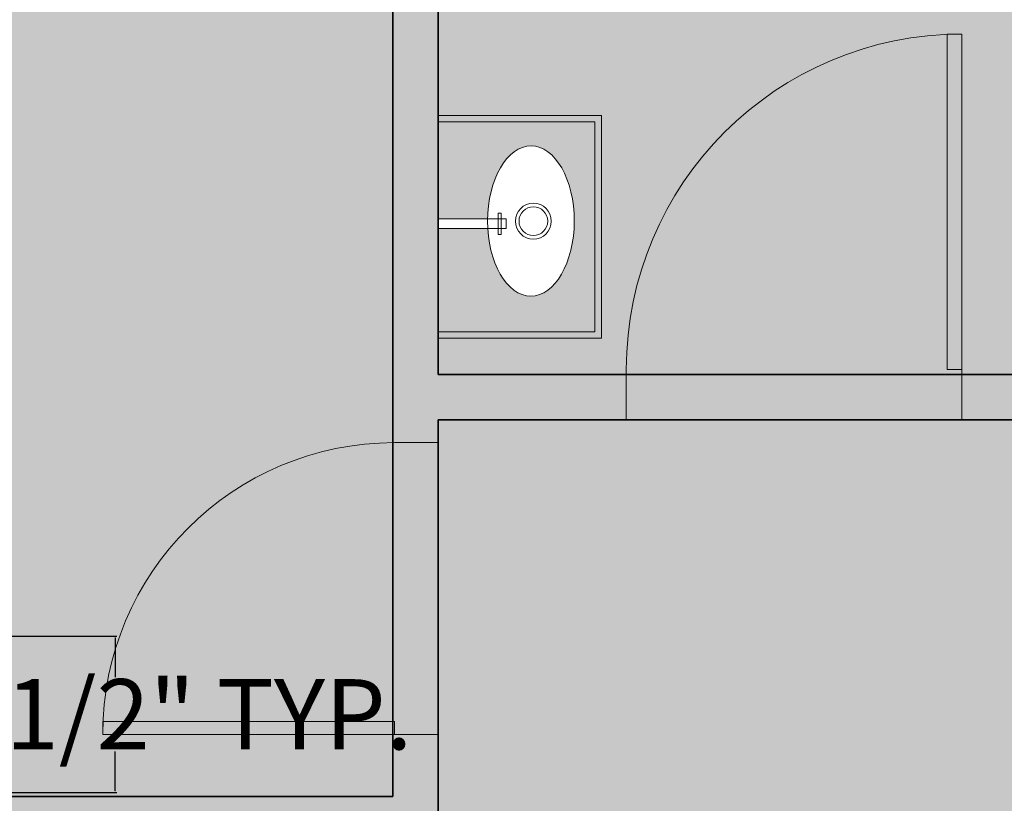
# Model space of a CAD drawing. Units: inches. Extents: x 1316 to 1777, y 813 to 1650.
# Tile 14 of 22: x 1469 to 1567, y 1434 to 1512. Entities that reach past the tile are written whole.
import ezdxf

# ---------------------------------------------------------------- set-up
doc = ezdxf.new("R2010")
doc.units = ezdxf.units.IN
doc.header["$MEASUREMENT"] = 0
for name, color, linetype, lineweight in [('A-ANNO-DIMS', 2, 'Continuous', 18), ('A-DOOR', 4, 'Continuous', 18), ('A-DOOR-PATT', 253, 'Continuous', 13), ('A-FLOR-FIXT', 8, 'Continuous', 18), ('A-FLOR-FIXT-PATT', 23, 'Continuous', 13), ('A-WALL-PATT', 250, 'Continuous', 13), ('walls', 250, 'Continuous', 35)]:
    doc.layers.add(name, color=color, linetype=linetype, lineweight=lineweight)
doc.layers.add('A-FLOR-PATT', color=254, linetype='Continuous', lineweight=13, true_color=0xfeeab9)
doc.styles.get("Standard").update_dxf_attribs({"font": 'arial.ttf'})
doc.dimstyles.get("Standard").update_dxf_attribs({"dimtxt": 7, "dimasz": 0.18, "dimexe": 0.18, "dimexo": 0.0625, "dimgap": 0.09, "dimtad": 0, "dimtih": 1, "dimtoh": 1, "dimzin": 0, "dimdsep": 46, "dimlunit": 3, "dimtxsty": 'Standard', "dimcen": 0.09, "dimadec": 0, "dimazin": 0, "dimtfac": 1, "dimtofl": 0, "dimtmove": 0, "dimatfit": 3, "dimfxl": 1, "dimtolj": 1, "dimtzin": 0, "dimarcsym": 0})

# ---------------------------------------------------------------- blocks, each defined once
blk = doc.blocks.new('*U15')
for p, q in [((0, 0), (-1e-16, -5.999999999999999)), ((40, -6e-16), (40, -6))]:
    blk.add_line(p, q)
blk.add_lwpolyline([(0, 0), (5.6e-15, 40), (1.750000000000007, 40), (1.749999999999998, -7e-16)], close=True)
blk.add_arc((0, 0), 40, 0, 90)
blk = doc.blocks.new('*D30')
at = {"layer": 'A-ANNO-DIMS', "color": 0, "lineweight": -2, "transparency": 16777216}
for p, q in [((1386.153353095512, 1434.699095169867), (1386.153353095512, 1422.57802783725)), ((1466.177135312958, 1434.699095169867), (1466.177135312958, 1422.57802783725)), ((1386.333353095512, 1422.75802783725), (1465.997135312959, 1422.75802783725)), ((1466.177135312958, 1422.75802783725), (1466.357135312958, 1422.75802783725))]:
    blk.add_line(p, q, dxfattribs=at)
at = {"layer": 'A-ANNO-DIMS', "color": 0, "transparency": 16777216}
for points in [[(1386.333353095512, 1422.78802783725), (1386.333353095512, 1422.72802783725), (1386.153353095512, 1422.75802783725)], [(1465.997135312959, 1422.78802783725), (1465.997135312959, 1422.72802783725), (1466.177135312958, 1422.75802783725)]]:
    blk.add_solid(points, dxfattribs=at)
at = {"layer": 'Defpoints', "color": 0, "transparency": 16777216}
for p in [(1386.153353095512, 1434.761595169867), (1466.177135312958, 1434.761595169867), (1466.177135312958, 1422.75802783725)]:
    blk.add_point(p, dxfattribs=at)
at = {"layer": 'A-ANNO-DIMS', "color": 0, "transparency": 16777216, "insert": (1518.078103935059, 1422.75802783725), "char_height": 7, "attachment_point": 5}
blk.add_mtext('\\A1;WARDROBE 6\'-8" TYP.', dxfattribs=at)
blk = doc.blocks.new('*D31')
at = {"layer": 'A-ANNO-DIMS', "color": 0, "lineweight": -2, "transparency": 16777216}
for p, q in [((1466.239635312959, 1450.329145456027), (1478.360702645576, 1450.329145456027)), ((1478.180702645576, 1450.149145456027), (1478.180702645576, 1446.257130203807)), ((1478.180702645576, 1434.941595169868), (1478.180702645576, 1438.833610422088)), ((1466.239635312959, 1434.761595169868), (1478.360702645576, 1434.761595169868))]:
    blk.add_line(p, q, dxfattribs=at)
at = {"layer": 'A-ANNO-DIMS', "color": 0, "transparency": 16777216}
for points in [[(1478.150702645576, 1450.149145456027), (1478.210702645576, 1450.149145456027), (1478.180702645576, 1450.329145456027)], [(1478.150702645576, 1434.941595169868), (1478.210702645576, 1434.941595169868), (1478.180702645576, 1434.761595169868)]]:
    blk.add_solid(points, dxfattribs=at)
at = {"layer": 'Defpoints', "color": 0, "transparency": 16777216}
for p in [(1466.177135312959, 1450.329145456027), (1478.180702645576, 1450.329145456027), (1466.177135312959, 1434.761595169868)]:
    blk.add_point(p, dxfattribs=at)
at = {"layer": 'A-ANNO-DIMS', "color": 0, "transparency": 16777216, "insert": (1478.180702645576, 1442.545370312947), "char_height": 7, "attachment_point": 5}
blk.add_mtext('\\A1;1\'-3 1/2" TYP.', dxfattribs=at)

msp = doc.modelspace()

# ---------------------------------------------------------------- hatches: boundary and pattern name
at = {"layer": 'A-DOOR-PATT'}
h = msp.add_hatch(color=256, dxfattribs=at)
h.dxf.hatch_style = 1
h.paths.add_polyline_path([(1440.064450217018, 1373.459281729462), (1411.195884528974, 1373.459281729462, 0.0109414287710455), (1411.168078720428, 1372.18876759644), (1440.064450217018, 1372.18876759644)])
h.paths.add_polyline_path([(1505.845136951899, 1441.821674157348), (1476.976571263855, 1441.821674157348, 0.0109414287710455), (1476.948765455309, 1440.551160024325), (1505.845136951899, 1440.551160024325)])
h.paths.add_polyline_path([(1510.345136951899, 1469.591483064839), (1505.989088495822, 1469.591483064839, 0.0012392441961977), (1505.845136951899, 1469.59112628206), (1505.845136951899, 1441.821674157348), (1505.989088495822, 1441.821674157348), (1505.989088495822, 1440.551160024325), (1510.345136951899, 1440.551160024325)])
at = {"layer": 'A-FLOR-FIXT-PATT'}
h = msp.add_hatch(color=256, dxfattribs=at)
h.dxf.hatch_style = 1
edge = h.paths.add_edge_path(flags=0)
edge.add_line((1525.946608831446, 1501.531624720906), (1510.345136951899, 1501.531624720906))
edge.add_line((1510.345136951899, 1501.531624720906), (1510.345136951899, 1491.869370531834))
edge.add_line((1510.345136951899, 1491.869370531834), (1515.276633424269, 1491.869370531834))
edge.add_ellipse((1519.58729945907, 1491.66311611605), major_axis=(0.0164125256646926, 7.480193534640648), ratio=0.5765346257282575, start_angle=99.88916701195939, end_angle=87.38634600921353, ccw=False)
edge.add_line((1515.294686933541, 1490.924472696575), (1510.345136951899, 1490.924472696575))
edge.add_line((1510.345136951899, 1490.924472696575), (1510.345136951899, 1480.628840110929))
edge.add_line((1510.345136951899, 1480.628840110929), (1525.946608831446, 1480.628840110929))
edge.add_line((1525.946608831446, 1480.628840110929), (1525.946608831446, 1501.531624720906))
h.paths.add_polyline_path([(1526.60513386119, 1502.15895166366), (1510.345136951899, 1502.15895166366), (1510.345136951899, 1501.531624720906), (1525.946608831446, 1501.531624720906), (1525.946608831446, 1480.628840110929), (1510.345136951899, 1480.628840110929), (1510.345136951899, 1480.003801757213), (1526.60513386119, 1480.003801757213)])
h = msp.add_hatch(color=256, dxfattribs=at)
h.dxf.hatch_style = 1
edge = h.paths.add_edge_path()
edge.add_line((1525.946608831446, 1501.531624720906), (1510.345136951899, 1501.531624720906))
edge.add_line((1510.345136951899, 1501.531624720906), (1510.345136951899, 1491.869370531834))
edge.add_line((1510.345136951899, 1491.869370531834), (1515.276633424269, 1491.869370531834))
edge.add_ellipse((1519.58729945907, 1491.66311611605), major_axis=(0.0164125256646926, 7.480193534640648), ratio=0.5765346257282575, start_angle=99.88916701195939, end_angle=87.38634600921353, ccw=False)
edge.add_line((1515.294686933541, 1490.924472696575), (1510.345136951899, 1490.924472696575))
edge.add_line((1510.345136951899, 1490.924472696575), (1510.345136951899, 1480.628840110929))
edge.add_line((1510.345136951899, 1480.628840110929), (1525.946608831446, 1480.628840110929))
edge.add_line((1525.946608831446, 1480.628840110929), (1525.946608831446, 1501.531624720906))
at = {"layer": 'A-FLOR-PATT'}
h = msp.add_hatch(color=256, dxfattribs=at)
h.dxf.hatch_style = 1
h.paths.add_polyline_path([(1704.173142217696, 1566.369300926962), (1574.845136951899, 1566.369300926962), (1574.845136951899, 1434.369300926962), (1704.173142217696, 1434.369300926962)])
h.paths.add_polyline_path([(1630.932461874496, 1542.855774057473), (1660.956030155827, 1542.855774057473), (1660.956030155827, 1535.715818603972), (1688.427101885747, 1535.715818603972), (1688.322102259768, 1546.60436195911), (1686.084685639232, 1547.859338051823), (1686.091126213631, 1547.880435327422), (1685.166410126033, 1550.96282228608), (1681.618706890439, 1555.397451330572), (1678.245560576594, 1552.474057858572), (1678.252731368384, 1552.432698816134), (1678.186671845043, 1552.423020957896), (1681.618706890439, 1555.397451330572), (1683.600958512701, 1556.058201871326), (1683.638878966592, 1556.171639211768), (1683.763607677471, 1556.112418259583), (1686.94026174383, 1557.171302948369), (1688.039438370375, 1558.584530039641), (1688.033686884187, 1558.6987426557), (1688.107680475544, 1558.672269889145), (1686.969155905838, 1557.208452585237), (1686.964873585789, 1557.179506895689), (1681.618706890439, 1555.397451330572), (1682.03945471648, 1554.871516548022), (1682.120272056126, 1554.846450938584), (1682.106618265419, 1554.787562111848), (1685.145085092905, 1550.989478577491), (1685.188096327656, 1550.976822603904), (1685.172977838666, 1550.940929910638), (1685.764092561596, 1548.97054750087), (1688.363951485033, 1547.81415954591), (1702.184723874646, 1547.81415954591), (1702.301389734572, 1535.715818603971), (1702.301389734572, 1481.715823291257), (1702.418055594498, 1469.617482349317), (1688.543767745673, 1469.617482349317), (1688.427101885747, 1481.715823291277), (1660.956030155827, 1481.715823291277), (1660.956030155827, 1470.852844465434), (1630.932461874496, 1470.852844465434)], flags=16)
h.paths.add_polyline_path([(1624.930620536026, 1450.279112811716), (1703.91936034353, 1450.279112810615), (1703.919360343335, 1436.319504549967), (1703.919360343529, 1435.026369171866), (1624.930620536164, 1435.026369171866), (1624.930620536164, 1435.468976146952)], flags=16)
h.paths.add_polyline_path([(1624.930620535934, 1443.713594124807), (1625.99502102627, 1443.713594124792), (1625.995021026347, 1449.228584792601), (1626.751763768497, 1449.228584792591), (1626.751763768421, 1443.713594124782), (1628.113786522866, 1443.713594124762), (1628.113786522943, 1449.228584792571), (1628.870529265094, 1449.228584792561), (1628.870529265016, 1443.713594124752), (1630.502206974044, 1443.713594124729), (1630.502206974121, 1449.228584792538), (1631.258949716271, 1449.228584792528), (1631.258949716194, 1443.713594124719), (1632.967677515695, 1443.713594124695), (1632.967677515771, 1449.228584792504), (1633.724420257922, 1449.228584792493), (1633.724420257845, 1443.713594124684), (1638.318139073099, 1443.71359412462), (1641.013180150264, 1449.599650991773), (1641.689053381981, 1449.290189808583), (1639.135704887691, 1443.713594124609), (1640.127645379921, 1443.713594124595), (1642.822686457085, 1449.599650991748), (1643.498559688802, 1449.290189808558), (1640.945211194512, 1443.713594124584), (1642.323321207278, 1443.713594124564), (1645.018362284442, 1449.599650991717), (1645.69423551616, 1449.290189808527), (1643.14088702187, 1443.713594124553), (1647.034868862889, 1443.713594124499), (1647.034868862966, 1449.228584792308), (1647.791611605116, 1449.228584792297), (1647.791611605039, 1443.713594124488), (1649.606344517206, 1443.713594124463), (1649.606344517283, 1449.228584792271), (1650.363087259433, 1449.228584792261), (1650.363087259356, 1443.713594124452), (1652.864535573064, 1443.713594124417), (1652.86453557314, 1449.228584792227), (1653.621278315291, 1449.228584792216), (1653.621278315213, 1443.713594124407), (1657.035058236599, 1443.713594124359), (1657.035058236676, 1449.228584792168), (1657.791800978826, 1449.228584792157), (1657.791800978749, 1443.713594124349), (1660.082736745753, 1443.713594124317), (1660.08273674583, 1449.228584792125), (1660.839479487981, 1449.228584792115), (1660.839479487904, 1443.713594124306), (1662.604942004505, 1443.713594124282), (1662.604942004582, 1449.228584792091), (1663.361684746731, 1449.22858479208), (1663.361684746655, 1443.713594124271), (1667.701933018638, 1443.71359412421), (1667.701933018715, 1449.228584792019), (1668.458675760865, 1449.228584792008), (1668.458675760788, 1443.7135941242), (1671.654902823707, 1443.713594124155), (1670.316094155395, 1449.228584791983), (1671.051478417664, 1449.407105279897), (1672.433624380832, 1443.713594124144), (1679.695593448107, 1443.713594124043), (1680.179092581217, 1449.2437371972), (1680.93295954233, 1449.177826782703), (1680.455222941554, 1443.713594124032), (1683.499753022321, 1443.71359412399), (1682.225483650305, 1448.723091425686), (1682.958871530074, 1448.909643819413), (1684.28059436644, 1443.713594123979), (1688.219132172317, 1443.713594123924), (1688.219132172395, 1449.228584791734), (1688.975874914544, 1449.228584791724), (1688.975874914468, 1443.713594123914), (1690.481907378039, 1443.713594123893), (1690.481907378116, 1449.228584791702), (1691.238650120266, 1449.228584791692), (1691.238650120189, 1443.713594123882), (1692.488012124579, 1443.713594123865), (1692.488012124656, 1449.228584791674), (1693.244754866807, 1449.228584791663), (1693.24475486673, 1443.713594123854), (1695.009222235677, 1443.71359412383), (1695.009222235755, 1449.228584791639), (1695.765964977904, 1449.228584791628), (1695.765964977828, 1443.713594123819), (1701.028667612474, 1443.713594123746), (1700.875476353593, 1443.379019460314), (1695.765964977823, 1443.379019460385), (1695.765964977718, 1435.871950703975), (1695.009222235568, 1435.871950703986), (1695.009222235673, 1443.379019460396), (1693.244754866725, 1443.379019460421), (1693.24475486662, 1435.87195070401), (1692.48801212447, 1435.871950704021), (1692.488012124574, 1443.379019460431), (1691.238650120184, 1443.379019460448), (1691.238650120079, 1435.871950704039), (1690.481907377929, 1435.871950704049), (1690.481907378034, 1443.379019460459), (1688.975874914463, 1443.37901946048), (1688.975874914358, 1435.871950704071), (1688.219132172208, 1435.871950704081), (1688.219132172313, 1443.379019460491), (1684.365700360234, 1443.379019460544), (1686.251552017633, 1435.965226900976), (1685.518164137864, 1435.778674507249), (1683.584859016115, 1443.379019460555), (1680.425971155915, 1443.379019460599), (1679.769629866386, 1435.871950704198), (1679.015762905273, 1435.937861118695), (1679.666341662468, 1443.37901946061), (1677.601704230459, 1443.379019460639), (1677.601704230349, 1435.459733534966), (1676.844961488199, 1435.459733534977), (1676.844961488309, 1443.379019460649), (1672.51484509118, 1443.37901946071), (1674.202394444223, 1436.427451881403), (1673.467010181954, 1436.248931393489), (1671.736123534055, 1443.379019460721), (1668.458675760783, 1443.379019460766), (1668.458675760679, 1435.871950704355), (1667.701933018528, 1435.871950704365), (1667.701933018633, 1443.379019460777), (1663.36168474665, 1443.379019460837), (1663.361684746545, 1435.871950704427), (1662.604942004395, 1435.871950704438), (1662.6049420045, 1443.379019460848), (1660.839479487899, 1443.379019460873), (1660.839479487794, 1435.871950704461), (1660.082736745644, 1435.871950704471), (1660.082736745749, 1443.379019460883), (1657.791800978744, 1443.379019460915), (1657.79180097864, 1435.871950704504), (1657.03505823649, 1435.871950704514), (1657.035058236594, 1443.379019460926), (1653.621278315209, 1443.379019460973), (1653.621278315104, 1435.871950704563), (1652.864535572954, 1435.871950704574), (1652.864535573059, 1443.379019460984), (1650.363087259352, 1443.379019461018), (1650.363087259247, 1435.871950704607), (1649.606344517097, 1435.871950704617), (1649.606344517201, 1443.379019461029), (1647.791611605034, 1443.379019461055), (1647.79161160493, 1435.871950704643), (1647.03486886278, 1435.871950704654), (1647.034868862884, 1443.379019461065), (1642.987695762989, 1443.379019461121), (1639.390427205708, 1435.522468600366), (1638.714553973992, 1435.831929783556), (1642.170129948397, 1443.379019461133), (1640.792019935631, 1443.379019461152), (1637.194751378351, 1435.522468600396), (1636.518878146634, 1435.831929783587), (1639.974454121039, 1443.379019461164), (1638.98251362881, 1443.379019461177), (1635.38524507153, 1435.522468600422), (1634.709371839813, 1435.831929783612), (1638.164947814218, 1443.379019461189), (1633.72442025784, 1443.379019461251), (1633.724420257736, 1435.87195070484), (1632.967677515585, 1435.87195070485), (1632.96767751569, 1443.379019461261), (1631.25894971619, 1443.379019461285), (1631.258949716085, 1435.871950704874), (1630.502206973934, 1435.871950704885), (1630.502206974039, 1443.379019461296), (1628.870529265012, 1443.379019461319), (1628.870529264907, 1435.871950704907), (1628.113786522757, 1435.871950704918), (1628.113786522861, 1443.379019461329), (1626.751763768416, 1443.379019461348), (1626.751763768311, 1435.871950704937), (1625.995021026161, 1435.871950704948), (1625.995021026265, 1443.379019461359), (1624.93062053593, 1443.379019461374)], flags=0)
h.paths.add_polyline_path([(1683.8388184438, 1491.516940873591), (1691.02243240811, 1491.516940873591), (1691.070762458724, 1491.582489532902), (1691.070762458724, 1529.618213888147), (1699.230602800613, 1529.618213888147), (1699.230602800613, 1513.795458682787), (1691.070762458724, 1513.795458682787), (1691.070762458724, 1507.339696078951), (1699.230602800613, 1507.339696078951), (1699.230602800613, 1491.516940873591), (1691.02243240811, 1491.516940873591), (1683.8388184438, 1481.774011611434)], flags=0)
h.paths.add_polyline_path([(1691.014795269945, 1475.340823211309, -1), (1699.947028070227, 1475.340823211309, -1)], flags=0)
h.paths.add_polyline_path([(1690.898129410018, 1541.439159465963, -1), (1699.830362210301, 1541.439159465963, -1)], flags=0)
h.paths.add_polyline_path([(1505.845136951899, 1469.59112628206), (1505.845136951899, 1566.369300926962), (1386.064450217018, 1566.369300926962), (1386.064450217018, 1450.329145456028), (1465.696913734326, 1450.329145454916), (1465.696913734311, 1449.245294229286), (1466.177135312148, 1449.025415810232), (1465.696913734293, 1447.976596354367), (1465.696913734127, 1436.054730552491), (1465.69691373438, 1434.369300926962), (1505.845136951899, 1434.369300926962), (1505.845136951899, 1440.551160024325), (1476.948765455309, 1440.551160024325), (1476.948765455309, 1441.821674157348), (1476.976571263855, 1441.821674157348, -0.4000144639257896)])
edge = h.paths.add_edge_path(flags=16)
edge.add_spline(control_points=[(1456.972809125729, 1471.793867521006), (1457.023168566332, 1471.720656303634), (1457.137927411569, 1471.553822942034), (1456.942290846074, 1471.24192378408), (1456.670432209587, 1470.85108586496), (1456.942844502639, 1470.632431111965), (1457.080784081584, 1470.521712376681)], knot_values=[0, 0, 0, 0, 0.3521435018204935, 0.802462877712905, 1.439322186147505, 2.092600477110673, 2.092600477110673, 2.092600477110673, 2.092600477110673], degree=3, periodic=0)
edge.add_spline(control_points=[(1457.32475547428, 1471.793867521006), (1457.375114914907, 1471.720656303634), (1457.489873760197, 1471.55382294204), (1457.294237194615, 1471.24192378409), (1457.022378558147, 1470.851085864945), (1457.294790851223, 1470.632431111962), (1457.432730430185, 1470.521712376681)], knot_values=[0, 0, 0, 0, 0.3521435018524344, 0.8024628777664833, 1.439322186201083, 2.092600477201539, 2.092600477201539, 2.092600477201539, 2.092600477201539], degree=3, periodic=0)
edge = h.paths.add_edge_path(flags=16)
edge.add_line((1429.512779258274, 1471.793867521006), (1429.512779258274, 1482.65684634685))
edge.add_line((1429.512779258274, 1482.65684634685), (1402.041707528354, 1482.65684634685))
edge.add_line((1402.041707528354, 1482.65684634685), (1401.925041668428, 1470.55850540489))
edge.add_line((1401.925041668428, 1470.55850540489), (1388.050753819603, 1470.55850540489))
edge.add_line((1388.050753819603, 1470.55850540489), (1388.167419679529, 1482.656846346828))
edge.add_line((1388.167419679529, 1482.656846346828), (1388.167419679529, 1536.656841659541))
edge.add_line((1388.167419679529, 1536.656841659541), (1388.284085539456, 1548.755182601482))
edge.add_line((1388.284085539456, 1548.755182601482), (1402.158373388281, 1548.755182601482))
edge.add_line((1402.158373388281, 1548.755182601482), (1402.041707528354, 1536.656841659544))
edge.add_line((1402.041707528354, 1536.656841659544), (1429.512779258274, 1536.656841659544))
edge.add_line((1429.512779258274, 1536.656841659544), (1429.512779258274, 1543.796797113046))
edge.add_line((1429.512779258274, 1543.796797113046), (1456.931962466967, 1543.796797113046))
edge.add_spline(control_points=[(1456.931962466967, 1543.796797113046), (1456.986865443904, 1543.874076116505), (1457.107876047541, 1544.044405293154), (1456.910861506863, 1544.361471057989), (1456.638392620445, 1544.752143549724), (1456.910896769912, 1544.97082320328), (1457.048882861572, 1545.081554547293)], knot_values=[0, 0, 0, 0, 0.3739942808350491, 0.8243136566734239, 1.461172965108024, 2.114451256071192, 2.114451256071192, 2.114451256071192, 2.114451256071192], degree=3, periodic=0)
edge.add_spline(control_points=[(1457.400829210173, 1545.081554547293), (1457.262843118497, 1544.970823203282), (1456.990338969004, 1544.752143549739), (1457.262807855405, 1544.361471057978), (1457.459822396166, 1544.044405293151), (1457.338811792485, 1543.874076116505), (1457.283908815528, 1543.796797113046)], knot_values=[0, 0, 0, 0, 0.6532782910004561, 1.290137599435056, 1.740456975295068, 2.114451256156171, 2.114451256156171, 2.114451256156171, 2.114451256156171], degree=3, periodic=0)
edge.add_line((1457.283908815528, 1543.796797113046), (1459.536347539605, 1543.796797113046))
edge.add_line((1459.536347539605, 1543.796797113046), (1459.536347539605, 1471.793867521006))
edge.add_line((1459.536347539605, 1471.793867521006), (1429.512779258274, 1471.793867521006))
h.paths.add_polyline_path([(1406.629990970302, 1482.715034667006), (1399.446377005991, 1492.457963929164), (1399.398046955377, 1492.457963929164), (1391.238206613488, 1492.457963929164), (1391.238206613488, 1508.280719134523), (1399.398046955377, 1508.280719134523), (1399.398046955377, 1514.736481738359), (1391.238206613488, 1514.736481738359), (1391.238206613488, 1530.559236943719), (1399.398046955377, 1530.559236943719), (1399.398046955377, 1492.523512588475), (1399.446377005991, 1492.457963929164), (1406.629990970302, 1492.457963929164)], flags=0)
h.paths.add_polyline_path([(1399.454014144157, 1476.281846266881, -1), (1390.521781343874, 1476.281846266881, -1)], flags=0)
h.paths.add_polyline_path([(1390.6384472038, 1542.380182521536, -1), (1399.570680004083, 1542.380182521536, -1)], flags=0)
h.paths.add_polyline_path([(1487.293056362471, 1548.286149051947), (1487.079502016331, 1548.251927299585), (1487.103569785383, 1547.964021870899)], flags=16)
h.paths.add_polyline_path([(1491.492982446476, 1552.843098273946), (1490.887177911646, 1552.654179820082), (1490.949131147825, 1552.371760481782)], flags=16)
h.paths.add_polyline_path([(1489.965856241701, 1554.409093477953), (1489.859237467603, 1554.560966855939), (1489.717595420028, 1554.444559309621)], flags=16)
h.paths.add_polyline_path([(1497.300520669187, 1546.483185317046), (1497.294080094788, 1546.462088041448), (1497.309433365481, 1546.453476329402)], flags=16)
h.paths.add_polyline_path([(1496.386147786754, 1549.55264326925), (1492.828101345996, 1554.000201320197), (1492.655191111377, 1554.938856879555), (1492.454253708313, 1555.029495446401), (1492.589458265089, 1555.295692330835), (1491.80635643937, 1559.546816527597), (1491.869344065012, 1559.506442238776), (1491.824003397901, 1559.45101875271), (1492.828101345996, 1554.000201320197), (1494.810352968258, 1554.660951860951), (1494.848273422149, 1554.774389201393), (1494.973002133028, 1554.715168249208), (1496.010177934814, 1555.060893516469), (1496.078408037368, 1555.314097280749), (1496.340636955742, 1555.171046523446), (1498.149656199386, 1555.774052937994), (1499.248832825931, 1557.187280029266), (1499.243081339744, 1557.301492645324), (1499.317074931101, 1557.275019878769), (1498.178550361395, 1555.811202574862), (1498.174268041345, 1555.782256885313), (1492.828101345996, 1554.000201320197), (1493.248849172036, 1553.474266537646), (1493.329666511683, 1553.449200928208), (1493.316012720976, 1553.390312101472), (1495.202682324877, 1551.031975096595), (1495.701629872663, 1550.956726846686), (1495.574163147194, 1550.5676240687), (1496.354479548461, 1549.592228567115), (1496.397490783212, 1549.579572593528)], flags=16)
h.paths.add_polyline_path([(1486.021260248876, 1555.224454602706), (1485.9580139158, 1555.548733897003), (1483.595005607934, 1557.911742204869), (1483.280309209078, 1557.859129136746), (1483.243224833943, 1558.26352297886), (1486.270024687331, 1555.236723125471)], flags=16)
h.paths.add_polyline_path([(1505.845136951899, 1469.59112628206, 0.4000144639257898), (1476.976571263855, 1441.821674157348), (1505.845136951899, 1441.821674157348)], flags=17)
h = msp.add_hatch(color=256, dxfattribs=at)
h.dxf.hatch_style = 1
h.paths.add_polyline_path([(1561.016280979732, 1510.242898591528), (1561.016280979732, 1510.274875060637), (1562.477362604382, 1510.274875060637), (1562.477362604382, 1476.87872364005), (1562.477362604382, 1471.869300926962), (1529.081211183796, 1471.869300926962), (1529.081211183796, 1476.87872364005, -0.4014527144963571)])
h.paths.add_polyline_path([(1570.345136951899, 1566.369300926962), (1510.345136951899, 1566.369300926962), (1510.345136951899, 1502.15895166366), (1526.60513386119, 1502.15895166366), (1526.60513386119, 1480.003801757213), (1510.345136951899, 1480.003801757213), (1510.345136951899, 1476.369300926962), (1529.081211183796, 1476.369300926962), (1529.081211183796, 1476.87872364005, -0.4014527144963572), (1561.016280979732, 1510.242898591528), (1561.016280979732, 1510.274875060637), (1562.477362604382, 1510.274875060637), (1562.477362604382, 1476.369300926962), (1570.345136951899, 1476.369300926962)])
h.paths.add_polyline_path([(1528.659165159676, 1540.981508023645), (1528.659165159676, 1542.824755921347), (1529.119977134102, 1552.040995409852), (1528.659165159676, 1552.040995409852), (1528.659165159676, 1553.884243307553), (1529.119964231426, 1553.884243307553, -0.2060810176159248), (1535.571344776055, 1559.041430427285), (1535.571344776055, 1561.257234898357), (1534.649720827205, 1561.257234898357), (1534.649720827205, 1562.178858847208), (1532.806472929504, 1562.178858847208), (1532.806472929504, 1563.100482796059), (1543.86596031571, 1563.100482796059), (1543.86596031571, 1562.178858847208), (1542.022712418009, 1562.178858847208), (1542.022712418009, 1561.257234898357), (1541.101088469158, 1561.257234898357), (1541.101088469158, 1559.041430427285, -0.2060810176159245), (1547.552469013788, 1553.884243307553), (1548.013268085538, 1553.884243307553), (1548.013268085538, 1552.040995409852), (1547.552456111112, 1552.040995409852), (1547.552456111112, 1542.824755921347), (1548.013268085538, 1542.824755921347), (1548.013268085538, 1540.981508023645)], flags=16)
h.paths.add_polyline_path([(1704.173142217696, 1429.869300926962), (1602.173142217695, 1429.869300926962), (1602.173142217695, 1408.281186528541), (1631.069513714286, 1408.281186528541), (1631.069513714286, 1407.010672395518), (1631.04170790574, 1407.010672395518, -0.4000144639257927), (1602.173142217695, 1379.241220270806), (1602.173142217696, 1369.869300926962), (1625.31012555338, 1369.869300926962), (1625.31012555338, 1385.783403917709), (1647.465275459828, 1385.783403917709), (1647.465275459828, 1369.869300926962), (1704.173142217696, 1369.869300926962)])
h.paths.add_polyline_path([(1669.736853868253, 1382.592842276831), (1670.236853868253, 1382.592842276831), (1670.236853868253, 1392.592842276831), (1669.736853868253, 1392.592842276831), (1669.736853868253, 1394.592842276831), (1690.736853868253, 1394.592842276831), (1690.736853868253, 1392.592842276831), (1690.236853868253, 1392.592842276831), (1690.236853868253, 1382.592842276831), (1690.736853868253, 1382.592842276831), (1690.736853868253, 1380.592842276831), (1690.236867868188, 1380.592842276831, -0.2060810176159203), (1683.236853868253, 1374.997081526295), (1683.236853868253, 1372.592842276831), (1684.236853868253, 1372.592842276831), (1684.236853868253, 1371.592842276831), (1686.236853868253, 1371.592842276831), (1686.236853868253, 1370.592842276831), (1674.236853868253, 1370.592842276831), (1674.236853868253, 1371.592842276831), (1676.236853868253, 1371.592842276831), (1676.236853868253, 1372.592842276831), (1677.236853868253, 1372.592842276831), (1677.236853868253, 1374.997081526295, -0.2060810176159203), (1670.236839868318, 1380.592842276831), (1669.736853868253, 1380.592842276831)], flags=16)
h.paths.add_polyline_path([(1631.04170790574, 1407.010672395518), (1602.029190673773, 1407.010672395518), (1602.029190673773, 1408.281186528541), (1597.673142217696, 1408.281186528541), (1597.673142217696, 1379.240863488028), (1602.029190673773, 1379.240863488028, 0.4014527144963568)])
h = msp.add_hatch(color=256, dxfattribs=at)
h.dxf.hatch_style = 1
h.paths.add_polyline_path([(1567.673142217696, 1281.369300926962), (1651.673142217696, 1281.369300926962), (1651.673142217696, 1365.369300926962), (1597.673142217696, 1365.369300926962), (1597.673142217696, 1429.869300926962), (1570.345136951899, 1429.869300926962), (1570.345136951899, 1471.869300926962), (1510.345136951899, 1471.869300926962), (1510.345136951899, 1429.869300926962), (1444.564450217018, 1429.869300926962), (1444.564450217018, 1322.882360660317), (1444.564450217018, 1300.087519887597), (1510.564450217018, 1300.087519887597), (1510.564450217018, 1295.093869264817), (1510.564450217018, 1240.869300926962), (1386.064450217018, 1240.869300926962), (1386.064450217018, 1171.184826128129), (1400.961298831769, 1171.184826128129), (1400.961298831769, 1106.74181853581), (1386.064450217018, 1106.74181853581), (1386.064450217018, 1072.869300926962), (1510.564450217018, 1072.869300926962), (1510.564450217018, 1040.172951843256), (1541.068383692007, 1040.172951843256, -0.367085007058701), (1572.764174999282, 1069.546549507821), (1572.764174999282, 1069.578525976929), (1574.225256623933, 1069.578525976929), (1574.225256623933, 1040.172951843256), (1616.037285953149, 1040.172951843256), (1616.037285953149, 1086.627161740109), (1616.037285953149, 1103.704513499145), (1613.066060418845, 1105.234780569291), (1616.037285953149, 1106.685539866415), (1616.037285953149, 1123.869300926962), (1567.673142217696, 1123.869300926962)])
h.paths.add_polyline_path([(1508.987494855724, 1198.018101264616), (1511.117481528599, 1198.018101264616), (1511.117481528599, 1200.148087937491), (1532.594847146751, 1200.148087937491), (1532.594847146751, 1198.018101264616), (1534.724833819626, 1198.018101264616), (1534.724833819626, 1176.008238978245), (1530.464860473877, 1176.008238978245), (1530.464860473877, 1176.71823453587), (1513.247468201473, 1176.71823453587), (1513.247468201473, 1176.008238978245), (1508.987494855724, 1176.008238978245)], flags=16)
h.paths.add_polyline_path([(1505.978911344017, 1151.314990471522), (1521.503967005494, 1151.314990471522), (1521.503967005494, 1123.622553675171), (1505.978911344017, 1123.622553675171)], flags=16)
h.paths.add_polyline_path([(1507.734238645614, 1150.100746953806, -1), (1506.932299902515, 1150.100746953806, -1)], flags=0)
h.paths.add_polyline_path([(1512.288074001727, 1138.353334368216), (1512.279600715468, 1138.392440283947), (1512.219350358134, 1138.376242249414)], flags=0)
h.paths.add_polyline_path([(1511.538708600003, 1138.926307509397), (1511.801586230713, 1138.967144364025), (1511.816822451641, 1139.269704188439), (1511.606794574277, 1139.246286533845)], flags=0)
h.paths.add_polyline_path([(1513.744555260512, 1140.234298321423), (1513.680232363733, 1139.885116881769), (1514.013725426534, 1140.045442118172), (1513.85452204526, 1140.307851476896)], flags=0)
h.paths.add_polyline_path([(1513.759454991183, 1139.088508933479), (1514.004707571892, 1139.255238426424), (1513.806733823314, 1139.482778214552), (1513.564128907831, 1139.327271464974)], flags=0)
h.paths.add_polyline_path([(1514.219475210051, 1138.385213274156), (1514.335730050378, 1138.330012877603), (1514.544443105969, 1138.319719602207), (1514.802071501717, 1138.873746829037), (1514.451386945615, 1138.715560522777)], flags=0)
h.paths.add_polyline_path([(1514.576784523415, 1137.439218133731), (1514.572807725035, 1137.400121795131), (1514.699202201671, 1137.400121795131), (1514.696265725507, 1137.401958254237)], flags=0)
h.paths.add_polyline_path([(1512.259630054145, 1136.199252443718), (1512.198645006043, 1136.399020086717), (1512.031969302785, 1136.324884611944), (1512.095408670439, 1136.101205019573), (1512.257489338984, 1136.192116726515)], flags=0)
h.paths.add_polyline_path([(1512.643663084783, 1137.273739653883), (1512.355504649132, 1137.230281342332), (1512.431954114942, 1137.048783229095), (1512.702875297586, 1137.092989450977)], flags=0)
h.paths.add_polyline_path([(1513.048588650928, 1137.592520798729), (1512.979298324136, 1137.799799709794), (1512.842806872769, 1137.757466697763), (1512.887278702865, 1137.556025839099)], flags=0)
h.paths.add_polyline_path([(1513.269281623239, 1138.555876366321), (1513.570749546786, 1137.962332598873), (1513.458764523686, 1136.814048268166), (1513.212081965274, 1137.877990637943), (1513.032322366809, 1138.442602014432)], flags=0)
h.paths.add_polyline_path([(1514.891020715756, 1136.377090047208), (1514.695899864911, 1136.400535518201), (1514.682939550409, 1136.245500587688), (1514.870369662043, 1136.165423867704)], flags=0)
h.paths.add_polyline_path([(1514.142311807212, 1137.292647657223), (1514.047049214511, 1136.74320071616), (1514.270411313405, 1136.750949401328), (1514.327746372416, 1137.265481105849)], flags=0)
h.paths.add_polyline_path([(1515.361925908058, 1138.975942407129), (1515.333738674027, 1138.638448296537), (1515.595602136156, 1138.588081597507), (1515.627104749056, 1138.931608018565)], flags=0)
h.paths.add_polyline_path([(1537.284795120854, 1177.912388692567), (1537.994790678479, 1177.912388692567), (1537.994790678479, 1195.129780964971), (1537.284795120854, 1195.129780964971), (1537.284795120854, 1199.38975431072), (1559.294657407225, 1199.38975431072), (1559.294657407225, 1197.259767637845), (1561.4246440801, 1197.259767637845), (1561.4246440801, 1175.782402019693), (1559.294657407225, 1175.782402019693), (1559.294657407225, 1173.652415346818), (1559.378615070445, 1173.652415346818), (1559.378615070445, 1171.514303738793), (1561.51672667847, 1171.514303738793), (1561.51672667847, 1098.818509065945), (1559.378615070445, 1098.818509065945), (1559.378615070445, 1096.68039745792), (1537.284795120854, 1096.68039745792), (1537.284795120854, 1100.95662067397), (1537.997498990196, 1100.95662067397), (1537.997498990196, 1169.376192130768), (1537.284795120854, 1169.376192130768), (1537.284795120854, 1173.652415346818)], flags=16)
h.paths.add_polyline_path([(1518.623279367581, 1345.565265318288), (1519.133216999197, 1345.479657117201), (1519.133247129367, 1345.484585273925), (1518.623292796693, 1345.567461813277)], flags=16)
h.paths.add_polyline_path([(1518.798043157878, 1374.150014517315), (1519.307980789494, 1374.064406316228), (1519.308010919664, 1374.069334472953), (1518.79805658699, 1374.152211012305)], flags=16)
h.paths.add_polyline_path([(1537.763945546351, 1413.501272593833), (1537.678419015976, 1412.991334462891), (1537.683273643974, 1412.991304782267), (1537.76615767817, 1413.501259069119)], flags=16)
h.paths.add_polyline_path([(1572.904903294898, 1373.821409718101), (1573.926762419731, 1373.974678074354), (1574.026627442758, 1390.308820473798), (1573.007147246318, 1390.474521481455), (1573.006718884663, 1390.474591095266)], flags=16)
h.paths.add_polyline_path([(1572.730139504601, 1345.236660519073), (1573.751998629434, 1345.389928875326), (1573.851863652461, 1361.72407127477), (1572.832383456021, 1361.889772282427), (1572.831955094366, 1361.889841896238)], flags=16)
h.paths.add_polyline_path([(1537.210658487583, 1322.64259197221), (1537.363943428096, 1321.620732745983), (1553.69808582754, 1321.520867722956), (1553.863838585734, 1322.540776390265)], flags=16)
h.paths.add_polyline_path([(1535.907853535946, 1331.328394679552), (1527.214399285865, 1331.381545435045), (1527.663791889487, 1404.885186232545), (1564.415612288236, 1404.660489930734), (1563.966219684615, 1331.156849133235), (1555.272745017813, 1331.210000013553), (1553.946716560728, 1323.050730714162), (1537.134020158137, 1323.153521560007)], flags=16)
h.paths.add_polyline_path([(1536.149948378398, 1336.502989385165), (1536.235164066325, 1337.571577967879), (1536.323287084786, 1338.628101895201), (1536.410786509507, 1339.662781903015), (1536.494625364907, 1340.6698173033), (1536.573878305868, 1341.65983134291), (1536.648126641431, 1342.647834135966), (1536.716972722469, 1343.648937760143), (1536.780017027388, 1344.677948027938), (1536.836830656389, 1345.749875115879), (1536.91349345135, 1347.47536960008), (1536.930181129876, 1348.082213381731), (1536.86671979596, 1346.313806322279), (1536.754065794645, 1344.188314997416), (1536.618602559507, 1342.21851898877), (1536.494625364906, 1340.669817303289), (1536.410786509508, 1339.662781903024), (1536.323287084785, 1338.628101895196), (1536.235164066325, 1337.571577967878), (1536.149948378398, 1336.502989385167), (1536.071202820108, 1335.432319400725), (1536.002480605875, 1334.369653419014), (1535.917201218224, 1332.754159960459), (1535.909282823342, 1332.307756473361), (1535.96435308899, 1333.780079645636), (1536.071202820108, 1335.432319400726)], flags=0)
h.paths.add_polyline_path([(1540.411728678358, 1338.345220732376), (1540.538507986221, 1339.036732867615), (1540.667450686668, 1339.758144792479), (1540.798139602249, 1340.51803480286), (1540.930104638842, 1341.324675241543), (1541.06290820131, 1342.186644529235), (1541.195663950278, 1343.109256879628), (1541.325751198274, 1344.084667215432), (1541.450112594895, 1345.102072455087), (1541.565699126105, 1346.150363189455), (1541.669432399664, 1347.218634373414), (1541.758274858692, 1348.295980712192), (1541.829158319786, 1349.371497098253), (1541.87902418423, 1350.434176273261), (1541.905658245644, 1351.475864398132), (1541.910264078201, 1352.499718972741), (1541.894848813054, 1353.511751165878), (1541.861450207875, 1354.517971959091), (1541.812104772023, 1355.524188157142), (1541.748831093802, 1356.536615043187), (1541.673675267255, 1357.560957271187), (1541.551221046702, 1359.062282646612), (1541.495486505545, 1359.670454934914), (1541.588655256529, 1358.603328035907), (1541.721318618915, 1356.976835527602), (1541.846114060333, 1354.980013725856), (1541.912433480836, 1352.981966815021), (1541.903299375855, 1350.951498912638), (1541.805645357175, 1348.870418133965), (1541.627733180341, 1346.712969607265), (1541.39605931794, 1344.611846225434), (1541.135168242209, 1342.655652549989), (1540.871929016276, 1340.947082961546), (1540.617179283622, 1339.465841984599), (1540.411728678363, 1338.345220732389), (1540.287580984743, 1337.67502977883), (1540.166494164132, 1337.01788791383), (1540.048925605183, 1336.365114503449), (1539.936674201221, 1335.710368832696), (1539.836864251217, 1335.055036635329), (1539.758020939376, 1334.402536924379), (1539.708629238703, 1333.756391050932), (1539.697173498044, 1333.120018277682), (1539.75093556766, 1332.162191347439), (1539.822087714565, 1331.89006440645), (1539.690956844971, 1332.774679737417), (1539.713650637448, 1334.035332547662), (1539.86680860596, 1335.30285325234), (1540.085210789094, 1336.576760560778), (1540.287580984743, 1337.67502977883)], flags=0)
h.paths.add_polyline_path([(1545.598581542273, 1331.583674047033), (1545.601408931398, 1331.616855477121), (1545.614142276281, 1331.689058908809), (1545.736718477884, 1332.197227143153), (1545.766951209007, 1332.331509735297), (1545.840044120643, 1332.681341212682), (1545.924609388668, 1333.114205605127), (1546.015565858785, 1333.613901317454), (1546.107830504227, 1334.163920489319), (1546.196310713542, 1334.747857411176), (1546.27592408412, 1335.349306311069), (1546.341588213349, 1335.951861417042), (1546.388220074462, 1336.539014868746), (1546.411904372759, 1337.098233262493), (1546.413511757999, 1337.631655211558), (1546.395048737181, 1338.145189796344), (1546.358553067975, 1338.644847998394), (1546.30606313221, 1339.136742887642), (1546.239595021565, 1339.626681393686), (1546.161196702551, 1340.120674435653), (1546.072884891005, 1340.624631031533), (1545.887738197254, 1341.63015699768), (1545.717659533451, 1342.62070013092), (1545.546853733249, 1343.94500888803), (1545.431881256549, 1345.533720124316), (1545.403899849759, 1347.401905451854), (1545.417510423816, 1348.013069267128), (1545.410556413592, 1346.957478372932), (1545.425070640934, 1345.988432507364), (1545.462877367243, 1345.105410056077), (1545.521092971858, 1344.300975918152), (1545.595702123642, 1343.566272620922), (1545.68263719895, 1342.892238827028), (1545.777872657803, 1342.270017126221), (1545.877351709551, 1341.690648207114), (1545.977037981224, 1341.145172633476), (1546.133225269608, 1340.296924301995), (1546.32712189736, 1339.07516870602), (1546.43378476773, 1337.614859053002), (1546.377188266119, 1336.278538916938), (1546.246417261819, 1335.078542247844), (1546.032296532176, 1333.665423983985), (1545.840044120643, 1332.681341212682), (1545.766951209007, 1332.331509735297)], flags=0)
h.paths.add_polyline_path([(1551.802739251137, 1337.655775652498), (1551.96257269545, 1338.249893918501), (1552.102195298518, 1338.801154932478), (1552.224958021371, 1339.338328209144), (1552.330696453755, 1339.864579612065), (1552.418402861907, 1340.377056720641), (1552.487067639598, 1340.872600849098), (1552.535672844225, 1341.34835963925), (1552.563199284875, 1341.801276556129), (1552.568639227787, 1342.228499179132), (1552.550972857889, 1342.626868884903), (1552.509678498417, 1342.994551203202), (1552.446288501197, 1343.33337442512), (1552.362792521005, 1343.646491244529), (1552.261208966661, 1343.936747902882), (1552.143557495304, 1344.207194818415), (1552.011836098078, 1344.460678357413), (1551.868075265113, 1344.700350964085), (1551.746105860759, 1344.881722683215), (1550.887297650741, 1346.05192221882), (1550.42788872704, 1347.125680184261), (1550.183287427721, 1348.353333686171), (1550.047936052465, 1349.632359022536), (1549.978096005541, 1351.223542107026), (1549.974102148838, 1353.140827975589), (1549.989226669163, 1353.748427546368), (1549.975058438592, 1352.681752708607), (1549.977087298692, 1351.70778065901), (1549.995607655661, 1350.824569845699), (1550.030618304039, 1350.026913573531), (1550.082058657804, 1349.309911787039), (1550.149928759809, 1348.668561967865), (1550.234168024029, 1348.097964060535), (1550.334775869163, 1347.593013458303), (1550.451691709185, 1347.148810105696), (1550.584412233058, 1346.759844100773), (1550.73038050297, 1346.418678345312), (1550.88655602074, 1346.117266144286), (1551.049909745336, 1345.847764917032), (1551.217401178577, 1345.602127968521), (1551.385990446439, 1345.372410692116), (1551.55262809021, 1345.150770631988), (1552.000038284146, 1344.537104232464), (1552.453505275841, 1343.494713960715), (1552.591463897673, 1342.266339273388), (1552.508711326437, 1340.904737898757), (1552.245597777252, 1339.367339734202), (1551.924893638995, 1338.101128644033), (1551.618511514029, 1336.984114361546), (1551.405674157756, 1336.200020283199), (1551.009764092749, 1334.698598399404), (1550.877399289293, 1334.154667887629), (1551.263664389663, 1335.676855458292), (1551.618511514027, 1336.984114361536)], flags=0)
h.paths.add_polyline_path([(1558.642358998526, 1348.348341932098), (1558.795153425402, 1348.811416841303), (1558.918173552255, 1349.215358215379), (1559.008026171039, 1349.574581801048), (1559.061298904339, 1349.903707646641), (1559.075825921932, 1350.214183320864), (1559.054343192669, 1350.505992096326), (1559.00083323259, 1350.775944766007), (1558.919250427844, 1351.021260663692), (1558.81356708563, 1351.238750644777), (1558.687756761463, 1351.425429741436), (1558.545793010855, 1351.578312985846), (1558.391628971643, 1351.694415535011), (1558.228764001313, 1351.771674150153), (1558.05869086465, 1351.812121548804), (1557.882428128411, 1351.81871217754), (1557.700994359352, 1351.79440048294), (1557.515397915392, 1351.742140973996), (1557.326668820441, 1351.665092211649), (1557.135793766425, 1351.566004652943), (1556.943823194933, 1351.44803673399), (1556.751584825563, 1351.314654529213), (1556.741969848742, 1351.307485185875), (1556.174649390243, 1350.878470713214), (1555.982386678774, 1350.741107061228), (1555.790208852573, 1350.61762743028), (1555.103431920574, 1350.247624890473), (1554.019478994433, 1350.696346369238), (1553.658410413117, 1351.73359972735), (1553.592207666961, 1352.861368347784), (1553.704659497418, 1354.248209262139), (1553.753119918252, 1354.656598557367), (1553.684819216316, 1354.00352392911), (1553.637913725648, 1353.425049987856), (1553.614699631385, 1352.917691559993), (1553.614827379228, 1352.476039895736), (1553.637249468889, 1352.094077959223), (1553.680938817757, 1351.765788589762), (1553.744858758541, 1351.485256777466), (1553.82798220863, 1351.246465361642), (1553.929261667735, 1351.043397306428), (1554.04767130156, 1350.870239627912), (1554.182026927633, 1350.721997047951), (1554.330490954936, 1350.598680801359), (1554.491077653114, 1350.501119766308), (1554.661792955443, 1350.430449148551), (1554.840661964566, 1350.387599852234), (1555.02568040492, 1350.373707145527), (1555.214873379145, 1350.389701932573), (1555.406255781046, 1350.436515179933), (1555.598153361026, 1350.514157123772), (1555.790208852573, 1350.61762743028), (1555.982386678773, 1350.741107061227), (1556.174649390244, 1350.878470713214), (1556.366961410069, 1351.02389934801), (1556.559285288865, 1351.171267662216), (1556.751584825563, 1351.314654529213), (1556.943823194933, 1351.44803673399), (1557.135793766425, 1351.566004652943), (1557.326668820441, 1351.665092211648), (1558.042515074605, 1351.95733685961), (1558.893728230531, 1351.316279335487), (1559.136865914879, 1350.089672795452), (1558.886015641058, 1349.086793457618), (1558.642358998525, 1348.348341932093), (1558.463193064356, 1347.811615590227), (1558.261048830942, 1347.186822068983), (1558.03933929985, 1346.459443408408), (1557.677450203418, 1345.174834336041), (1557.548968991007, 1344.635807724703), (1557.908545731516, 1346.030339390738), (1558.328508124364, 1347.408140702653)], flags=0)
h.paths.add_polyline_path([(1562.145123345359, 1353.919129120074), (1562.250304117219, 1354.679787637482), (1562.34093833006, 1355.343853771733), (1562.416101040585, 1355.923686334763), (1562.475035862508, 1356.430826370303), (1562.517611688201, 1356.872216949942), (1562.54387555173, 1357.25388122627), (1562.553854069482, 1357.581842476714), (1562.547593651368, 1357.862021765479), (1562.525120913776, 1358.10044236999), (1562.486482890773, 1358.30312744284), (1562.431704950433, 1358.475896084676), (1562.361155192264, 1358.623850655281), (1562.276503898586, 1358.748001864806), (1562.179752001843, 1358.848337479786), (1562.072869183806, 1358.924743365611), (1561.957877418753, 1358.977309252376), (1561.836746388454, 1359.005921005473), (1561.71148785835, 1359.010668417409), (1561.584092552045, 1358.991539317136), (1561.456045120288, 1358.949239273116), (1561.341584300566, 1358.895014406292), (1560.779829007024, 1358.553784684453), (1560.630616275888, 1358.472819004295), (1560.474487483611, 1358.402819474164), (1560.311154867376, 1358.348484094885), (1559.637466910391, 1358.206630908504), (1558.973121038646, 1358.903907683205), (1558.815552073528, 1360.002456271339), (1558.803942930122, 1361.236291863163), (1558.829841213422, 1361.673699707903), (1558.80694301689, 1360.917438550413), (1558.812784665874, 1360.296580130481), (1558.845278068372, 1359.795210830316), (1558.902335132382, 1359.397417032129), (1558.981856932905, 1359.087183092155), (1559.081756002095, 1358.848697480995), (1559.199942999639, 1358.66584240408), (1559.334180223548, 1358.524951186848), (1559.481597784608, 1358.420834672959), (1559.639186392453, 1358.350550586885), (1559.803946965561, 1358.311156590683), (1559.97287021357, 1358.299710408824), (1560.142945597805, 1358.313065589002), (1560.311154867377, 1358.348484094885), (1560.474487483611, 1358.402819474164), (1560.630616275888, 1358.472819004295), (1560.779829007024, 1358.553784684454), (1560.923096183733, 1358.640810155187), (1561.061387688574, 1358.728886968651), (1561.195663195268, 1358.813006739421), (1561.382100208996, 1358.919625179564), (1561.341584300566, 1358.895014406292), (1561.972476451099, 1359.193894345525), (1562.53631106285, 1358.366963698877), (1562.559911530188, 1357.31074636116), (1562.455247211757, 1356.225674176933), (1562.323097858171, 1355.206225864646), (1562.145123345359, 1353.91912912008), (1562.026320333625, 1353.049417319218), (1561.815039989057, 1351.456922136686), (1561.751502783429, 1350.932786338753), (1561.948339842468, 1352.478551712307)], flags=0)
h.paths.add_polyline_path([(1572.764174999282, 1069.546549507821, 0.3670850070587006), (1541.068383692007, 1040.172951843256), (1572.764174999282, 1040.172951843256)], flags=17)
h.paths.add_polyline_path([(1572.764174999282, 1040.172951843256), (1541.068383692007, 1040.172951843256, 0.0299535364659094), (1540.829105203347, 1036.182374556343), (1540.829105203347, 1031.172951843255), (1574.225256623933, 1031.172951843255), (1574.225256623933, 1036.182374556343), (1572.764174999282, 1036.182374556343)])
at = {"layer": 'A-WALL-PATT'}
h = msp.add_hatch(color=256, dxfattribs=at)
h.dxf.hatch_style = 1
h.paths.add_polyline_path([(1713.173142217696, 1281.369300926962), (1656.173142217696, 1281.369300926962), (1656.173142217696, 1298.257717658217), (1651.673142217696, 1298.257717658217), (1651.673142217696, 1281.369300926962), (1567.673142217696, 1281.369300926962), (1567.673142217696, 1266.995117174766), (1572.173142217695, 1266.995117174766), (1572.173142217695, 1276.869300926963), (1704.173142217696, 1276.869300926962), (1704.173142217696, 1132.869300926962), (1608.640148269009, 1132.869300926962), (1608.640148269009, 1123.869300926962), (1704.173142217696, 1123.869300926962), (1704.173142217696, 1040.172951843256), (1652.868762127258, 1040.172951843256), (1652.868762127258, 1031.172951843254), (1713.173142217696, 1031.172951843253), (1713.173142217696, 1040.172951843256)])
h.paths.add_polyline_path([(1572.173142217696, 1237.954794134253), (1567.673142217696, 1237.954794134253), (1567.673142217696, 1123.869300926962), (1583.145592691861, 1123.869300926962), (1583.145592691861, 1132.869300926963), (1572.173142217696, 1132.869300926963)], flags=17)
h.paths.add_polyline_path([(1510.345136951899, 1566.369300926962), (1524.170902149835, 1566.369300926962), (1524.170902149835, 1571.984613741441), (1524.170902149835, 1575.369300926961), (1445.954793584458, 1575.369300926961), (1445.954793584458, 1566.369300926962), (1505.845136951899, 1566.369300926962), (1505.845136951899, 1469.591483064839), (1510.345136951899, 1469.591483064839), (1510.345136951899, 1471.869300926962), (1529.081211183796, 1471.869300926962), (1529.081211183796, 1476.369300926962), (1510.345136951899, 1476.369300926962)])
h.paths.add_polyline_path([(1609.722471703215, 1575.369300926961), (1545.118796217357, 1575.369300926961), (1545.118796217357, 1566.369300926962), (1570.345136951899, 1566.369300926962), (1570.345136951899, 1476.369300926962), (1562.477362604382, 1476.369300926962), (1562.477362604382, 1471.869300926962), (1570.345136951899, 1471.869300926962), (1570.345136951899, 1469.591483064839), (1574.845136951899, 1469.591483064839), (1574.845136951899, 1566.369300926962), (1609.722471703215, 1566.369300926962)])
h.paths.add_polyline_path([(1713.173142217696, 1575.369300926961), (1655.232651300773, 1575.369300926961), (1655.232651300773, 1566.369300926962), (1704.173142217696, 1566.369300926962), (1704.173142217696, 1434.369300926962), (1574.845136951899, 1434.369300926962), (1574.845136951899, 1440.551160024325), (1574.701185407976, 1440.551160024325), (1570.345136951899, 1440.551160024325), (1570.345136951899, 1429.869300926962), (1597.673142217696, 1429.869300926962), (1597.673142217696, 1408.281186528541), (1602.173142217695, 1408.281186528541), (1602.173142217695, 1429.869300926962), (1704.173142217696, 1429.869300926962), (1704.173142217696, 1410.703982852585), (1707.374745037781, 1410.703982852585), (1713.173142217696, 1410.703982852585)])
h.paths.add_polyline_path([(1713.173142217696, 1383.675544097327), (1704.173142217696, 1383.675544097327), (1704.173142217696, 1369.869300926962), (1602.173142217696, 1369.869300926962), (1602.173142217695, 1379.240863488028), (1597.673142217696, 1379.240863488028), (1597.673142217696, 1365.369300926962), (1713.173142217696, 1365.369300926962)])
h.paths.add_polyline_path([(1444.564450217018, 1429.869300926962), (1510.345136951899, 1429.869300926962), (1510.345136951899, 1440.551160024325), (1505.845136951899, 1440.551160024325), (1505.845136951899, 1434.369300926962), (1386.064450217018, 1434.369300926961), (1386.064450217018, 1566.369300926962), (1400.4446139869, 1566.369300926962), (1400.4446139869, 1575.369300926961), (1377.064450217018, 1575.369300926961), (1377.064450217018, 1412.813262305812), (1380.508552477466, 1412.813262305812), (1386.064450217018, 1412.813262305812), (1386.064450217018, 1429.869300926962), (1440.064450217018, 1429.869300926962), (1440.064450217018, 1401.229090636953), (1444.564450217018, 1401.229090636953)])
h.paths.add_polyline_path([(1444.564450217018, 1372.18876759644), (1440.064450217018, 1372.18876759644), (1440.064450217018, 1369.869300926962), (1386.064450217018, 1369.869300926962), (1386.064450217018, 1378.757622609401), (1377.064450217018, 1378.757622609401), (1377.064450217018, 1349.201183977028), (1381.117947355797, 1349.201183977028), (1386.064450217018, 1349.201183977028), (1386.064450217018, 1365.369300926962), (1440.064450217018, 1365.369300926962), (1440.064450217018, 1322.882360660317), (1444.564450217018, 1322.882360660317)])
h.paths.add_polyline_path([(1510.564450217018, 1295.093869264817), (1506.064450217018, 1295.093869264817), (1506.064450217018, 1245.369300926962), (1386.064450217018, 1245.369300926962), (1386.064450217018, 1272.58216425724), (1377.064450217018, 1272.58216425724), (1377.064450217018, 1212.904590025772), (1380.100240558029, 1212.904590025772), (1386.064450217018, 1212.904590025772), (1386.064450217018, 1240.869300926962), (1510.564450217018, 1240.869300926962)])
h.paths.add_polyline_path([(1386.064450217018, 1163.761289951094), (1377.064450217018, 1163.761289951094), (1377.064450217018, 1063.869300926961), (1419.36334498438, 1063.869300926961), (1419.36334498438, 1072.869300926962), (1386.064450217018, 1072.869300926962)])
h.paths.add_polyline_path([(1510.564450217018, 1072.869300926962), (1469.381492401113, 1072.869300926962), (1469.381492401113, 1063.869300926961), (1501.564450217018, 1063.869300926962), (1501.564450217018, 1033.022564166395), (1501.564450217018, 1031.172951843256), (1540.829105203347, 1031.172951843255), (1540.829105203347, 1036.182374556343, -0.0299535364659092), (1541.068383692007, 1040.172951843256), (1510.564450217018, 1040.172951843256)])
h.paths.add_polyline_path([(1607.368796217357, 1040.172951843256), (1574.225256623933, 1040.172951843256), (1574.225256623933, 1036.182374556343), (1574.225256623933, 1031.172951843255), (1607.368796217357, 1031.172951843254)], flags=17)
h.paths.add_polyline_path([(1637.054389108292, 1040.172951843256), (1624.70577568894, 1040.172951843256), (1624.70577568894, 1031.172951843254), (1637.054389108293, 1031.172951843254)], flags=17)

# ---------------------------------------------------------------- linework, layer by layer
at = {"layer": 'A-FLOR-FIXT'}
for p, q in [((1510.345136951899, 1502.15895166366), (1526.60513386119, 1502.15895166366)), ((1526.60513386119, 1502.15895166366), (1526.60513386119, 1480.003801757213)), ((1510.345136951899, 1501.531624720906), (1525.946608831446, 1501.531624720906)), ((1525.946608831446, 1501.531624720906), (1525.946608831446, 1480.628840110929)), ((1516.318672584757, 1492.44657464661), (1516.318672584757, 1490.322474452297)), ((1516.614103708012, 1492.44657464661), (1516.318672584757, 1492.44657464661)), ((1516.614103708012, 1490.322474452297), (1516.614103708012, 1492.44657464661)), ((1517.111098957315, 1491.869370531834), (1510.345136951899, 1491.869370531834)), ((1517.111098957315, 1491.869370531834), (1517.111098957315, 1490.924472696575)), ((1517.111098957315, 1490.924472696575), (1510.345136951899, 1490.924472696575)), ((1516.318672584757, 1490.322474452297), (1516.614103708012, 1490.322474452297)), ((1525.946608831446, 1480.628840110929), (1510.345136951899, 1480.628840110929)), ((1526.60513386119, 1480.003801757213), (1510.345136951899, 1480.003801757213))]:
    msp.add_line(p, q, dxfattribs=at)
for radius in [1.786721855987963, 1.786721855987973, 1.426627914243592, 1.426627914243628, 1.42662769250472, 1.426627377330596]:
    msp.add_circle((1519.826008708984, 1491.646758942555), radius, dxfattribs=at)
at = {"layer": 'A-FLOR-FIXT', "extrusion": (0, 0, -1)}
msp.add_ellipse((1519.58729945907, 1491.66311611605), major_axis=(0.0164125256646926, 7.480193534640648), ratio=0.5765346257282574, dxfattribs=at)
at = {"layer": 'walls'}
for p, q in [((1505.845136951899, 1566.369300926962), (1505.845136951899, 1434.369300926962)), ((1510.345136951899, 1566.369300926962), (1510.345136951899, 1476.369300926961)), ((1510.345136951899, 1476.369300926962), (1570.345136951899, 1476.369300926962)), ((1510.345136951899, 1471.869300926962), (1570.345136951899, 1471.869300926962)), ((1510.345136951899, 1471.869300926962), (1510.345136951899, 1429.869300926962)), ((1386.064450217018, 1434.369300926961), (1505.845136951899, 1434.369300926962))]:
    msp.add_line(p, q, dxfattribs=at)

# ---------------------------------------------------------------- block references
at = {"layer": 'A-DOOR', "xscale": -0.834903785514655, "yscale": 0.834903785514655, "zscale": 0.834903785514655}
msp.add_blockref('*U15', (1562.477362604382, 1476.87872364005), dxfattribs=at)
at = {"layer": 'A-DOOR', "xscale": 0.7260080760128325, "yscale": 0.7260080760128325, "zscale": 0.7260080760128325, "rotation": 90}
msp.add_blockref('*U15', (1505.989088495822, 1440.551160024325), dxfattribs=at)

# ---------------------------------------------------------------- dimensions: what is measured, and where the dimension line sits
at = {"layer": 'A-ANNO-DIMS'}
dim = msp.add_linear_dim(base=(1478.180702645576, 1450.329145456027), p1=(1466.177135312958, 1434.761595169867), p2=(1466.177135312958, 1450.329145456026), angle=90, text='<> TYP.', dimstyle='Standard', override={"dimdec": 1, "dimlfac": 1, "dimrnd": 0, "dimzin": 1, "dimdsep": 46, "dimlunit": 4, "dimfrac": 2}, dxfattribs=at)
dim.commit()
dim.dimension.update_dxf_attribs({"geometry": '*D31', "text_midpoint": (1478.180702645576, 1442.545370312947)})
dim = msp.add_linear_dim(base=(1466.177135312958, 1422.75802783725), p1=(1386.153353095512, 1434.761595169867), p2=(1466.177135312958, 1434.761595169867), text='WARDROBE <> TYP.', dimstyle='Standard', override={"dimdec": 1, "dimlfac": 1, "dimrnd": 0, "dimzin": 1, "dimdsep": 46, "dimlunit": 4, "dimfrac": 2}, dxfattribs=at)
dim.commit()
dim.dimension.update_dxf_attribs({"geometry": '*D30', "text_midpoint": (1518.078103935059, 1422.75802783725)})

doc.saveas('drawing.dxf')
